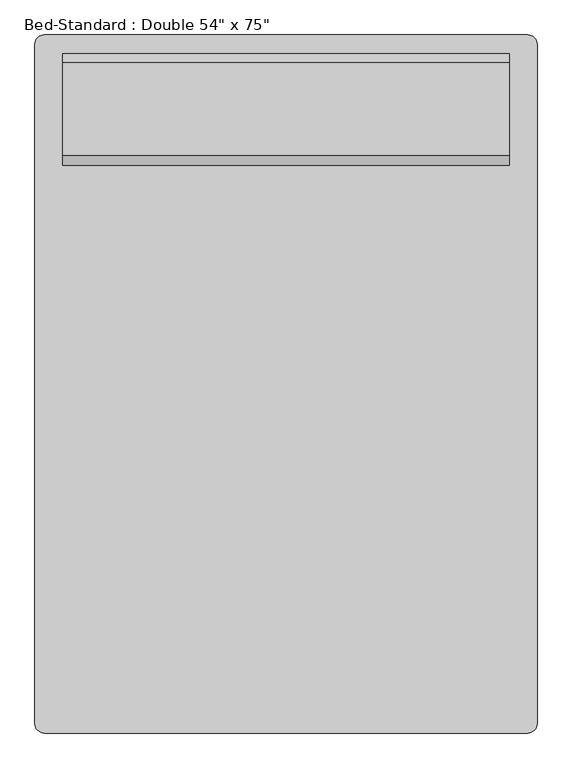
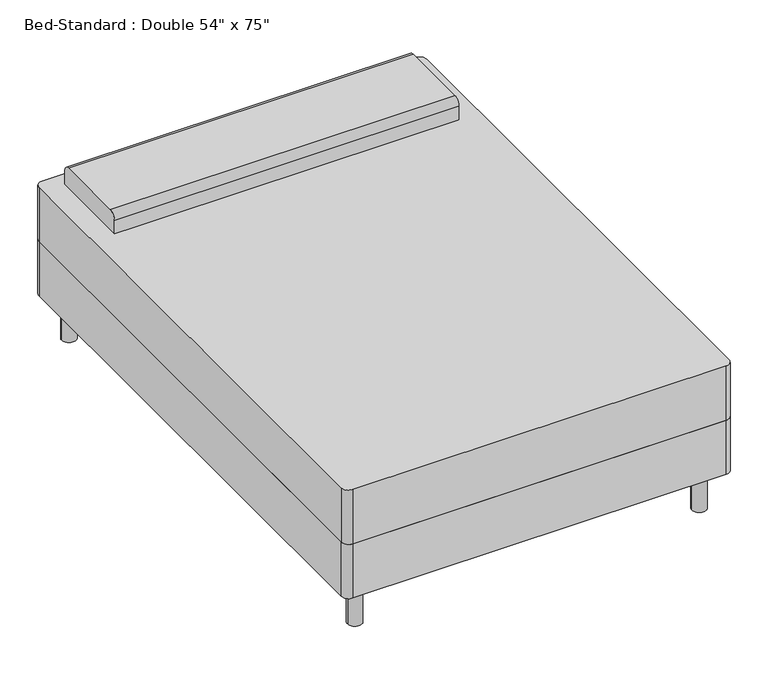
"""IFC4 building model written with IfcOpenShell, lengths in millimetres: furniture geometry."""

from ifc_helpers import new_model, si_unit, point, frame, frame_2d, origin, origin_with_axes, place, context, project, spatial, polyline, circle_curve, trimmed, segment, composite_curve, outline, extrude, source, transform, mapped, element, save


def furniture_52ef1662(model_context):
    return source(origin(), model_context, "Body", "SweptSolid", [
        extrude(outline(composite_curve([segment(polyline([(-388.9114754, 906.904918), (931.8885246, 906.904918)]), True, "CONTINUOUS"), segment(trimmed(circle_curve(frame_2d((931.8885246, 881.504918)), 25.4), [point((931.8885246, 906.904918))], [point((957.2885246, 881.504918))], False, "CARTESIAN"), True, "CONTINUOUS"), segment(polyline([(957.2885246, 881.504918), (957.2885246, -972.695082)]), True, "CONTINUOUS"), segment(trimmed(circle_curve(frame_2d((931.8885246, -972.695082)), 25.4), [point((957.2885246, -972.695082))], [point((931.8885246, -998.095082))], False, "CARTESIAN"), True, "CONTINUOUS"), segment(polyline([(931.8885246, -998.095082), (-388.9114754, -998.095082)]), True, "CONTINUOUS"), segment(trimmed(circle_curve(frame_2d((-388.9114754, -972.695082)), 25.4), [point((-388.9114754, -998.095082))], [point((-414.3114754, -972.695082))], False, "CARTESIAN"), True, "CONTINUOUS"), segment(polyline([(-414.3114754, -972.695082), (-414.3114754, 881.504918)]), True, "CONTINUOUS"), segment(trimmed(circle_curve(frame_2d((-388.9114754, 881.504918)), 25.4), [point((-414.3114754, 881.504918))], [point((-388.9114754, 906.904918))], False, "CARTESIAN"), True, "CONTINUOUS")], self_intersect=False)), frame((0.0, 0.0, 355.6), z_axis=(0.0, 0.0, 1.0), x_axis=(1.0, 0.0, 0.0)), (0.0, 0.0, 1.0), 203.2),
        extrude(outline(composite_curve([segment(trimmed(circle_curve(frame_2d((-338.1114754, 830.704918)), 25.4), [point((-363.5114754, 830.704918))], [point((-312.7114754, 830.704918))], False, "CARTESIAN"), True, "CONTINUOUS"), segment(trimmed(circle_curve(frame_2d((-338.1114754, 830.704918)), 25.4), [point((-312.7114754, 830.704918))], [point((-363.5114754, 830.704918))], False, "CARTESIAN"), True, "CONTINUOUS")], self_intersect=False)), origin_with_axes(), (0.0, 0.0, 1.0), 152.4),
        extrude(outline(composite_curve([segment(trimmed(circle_curve(frame_2d((881.0885246, 830.704918)), 25.4), [point((855.6885246, 830.704918))], [point((906.4885246, 830.704918))], False, "CARTESIAN"), True, "CONTINUOUS"), segment(trimmed(circle_curve(frame_2d((881.0885246, 830.704918)), 25.4), [point((906.4885246, 830.704918))], [point((855.6885246, 830.704918))], False, "CARTESIAN"), True, "CONTINUOUS")], self_intersect=False)), origin_with_axes(), (0.0, 0.0, 1.0), 152.4),
        extrude(outline(composite_curve([segment(trimmed(circle_curve(frame_2d((881.0885246, -921.895082)), 25.4), [point((855.6885246, -921.895082))], [point((906.4885246, -921.895082))], False, "CARTESIAN"), True, "CONTINUOUS"), segment(trimmed(circle_curve(frame_2d((881.0885246, -921.895082)), 25.4), [point((906.4885246, -921.895082))], [point((855.6885246, -921.895082))], False, "CARTESIAN"), True, "CONTINUOUS")], self_intersect=False)), origin_with_axes(), (0.0, 0.0, 1.0), 152.4),
        extrude(outline(composite_curve([segment(trimmed(circle_curve(frame_2d((-338.1114754, -921.895082)), 25.4), [point((-363.5114754, -921.895082))], [point((-312.7114754, -921.895082))], False, "CARTESIAN"), True, "CONTINUOUS"), segment(trimmed(circle_curve(frame_2d((-338.1114754, -921.895082)), 25.4), [point((-312.7114754, -921.895082))], [point((-363.5114754, -921.895082))], False, "CARTESIAN"), True, "CONTINUOUS")], self_intersect=False)), origin_with_axes(), (0.0, 0.0, 1.0), 152.4),
        extrude(outline(composite_curve([segment(polyline([(551.304918, 558.8), (551.304918, 609.6)]), True, "CONTINUOUS"), segment(trimmed(circle_curve(frame_2d((576.704918, 609.6)), 25.4), [point((551.304918, 609.6))], [point((576.704918, 635.0))], False, "CARTESIAN"), True, "CONTINUOUS"), segment(polyline([(576.704918, 635.0), (830.704918, 635.0)]), True, "CONTINUOUS"), segment(trimmed(circle_curve(frame_2d((830.704918, 609.6)), 25.4), [point((830.704918, 635.0))], [point((856.104918, 609.6))], False, "CARTESIAN"), True, "CONTINUOUS"), segment(polyline([(856.104918, 609.6), (856.104918, 558.8), (551.304918, 558.8)]), True, "CONTINUOUS")], self_intersect=False)), frame((-338.1114754, 0.0, 0.0), z_axis=(1.0, 0.0, 0.0), x_axis=(0.0, 1.0, 0.0)), (0.0, 0.0, 1.0), 1219.2),
        extrude(outline(composite_curve([segment(polyline([(-414.3114754, -972.695082), (-414.3114754, 881.504918)]), True, "CONTINUOUS"), segment(trimmed(circle_curve(frame_2d((-388.9114754, 881.504918)), 25.4), [point((-414.3114754, 881.504918))], [point((-388.9114754, 906.904918))], False, "CARTESIAN"), True, "CONTINUOUS"), segment(polyline([(-388.9114754, 906.904918), (931.8885246, 906.904918)]), True, "CONTINUOUS"), segment(trimmed(circle_curve(frame_2d((931.8885246, 881.504918)), 25.4), [point((931.8885246, 906.904918))], [point((957.2885246, 881.504918))], False, "CARTESIAN"), True, "CONTINUOUS"), segment(polyline([(957.2885246, 881.504918), (957.2885246, -972.695082)]), True, "CONTINUOUS"), segment(trimmed(circle_curve(frame_2d((931.8885246, -972.695082)), 25.4), [point((957.2885246, -972.695082))], [point((931.8885246, -998.095082))], False, "CARTESIAN"), True, "CONTINUOUS"), segment(polyline([(931.8885246, -998.095082), (-388.9114754, -998.095082)]), True, "CONTINUOUS"), segment(trimmed(circle_curve(frame_2d((-388.9114754, -972.695082)), 25.4), [point((-388.9114754, -998.095082))], [point((-414.3114754, -972.695082))], False, "CARTESIAN"), True, "CONTINUOUS")], self_intersect=False)), frame((0.0, 0.0, 152.4), z_axis=(0.0, 0.0, 1.0), x_axis=(1.0, 0.0, 0.0)), (0.0, 0.0, 1.0), 203.2),
    ])


if __name__ == "__main__":
    model = new_model("IFC4")
    model_context = context("Model", 3, world=origin())
    ifc_project = project(units=[si_unit("LENGTHUNIT", "METRE", prefix="MILLI")], contexts=[model_context])
    site = spatial("IfcSite", under=ifc_project)
    building = spatial("IfcBuilding", under=site)
    placement = place(None, origin())
    furniture_shape = furniture_52ef1662(model_context)
    element("IfcFurniture", 1, ObjectType="Bed-Standard : Double 54\" x 75\"", at=placement, inside=building, context=model_context, shape_type="MappedRepresentation", body=[
        mapped(furniture_shape, transform((0.0, 0.0, 0.0), x_axis=(1.0, 0.0, 0.0), y_axis=(0.0, 1.0, 0.0), z_axis=(0.0, 0.0, 1.0))),
    ])
    save(model, "model.ifc")

# Revit data of these elements
# Type "Bed-Standard : Double 54\" x 75\""
#   Assembly Code = "E2020200"
#   Length = 6' - 3"
#   Width = 4' - 6"
#   Leg Material = Steel, Chrome Plated
#   Mattress Material = Linen, White
#   Default Elevation = 0
# Element 1 (IfcFurniture, "Bed-Standard : Double 54\" x 75\"")
#   Materials on its faces: "Linen, White", "Steel, Chrome Plated"
# Materials
#   "Steel, Chrome Plated": class "Metal", colour RGB 17 17 17, transparency 0, Description = "Chromiuim plated steel", Cost = 0
#   "Linen, White": class "Textile", colour RGB 247 247 239, transparency 0, Description = "Linen, white", Cost = 0
